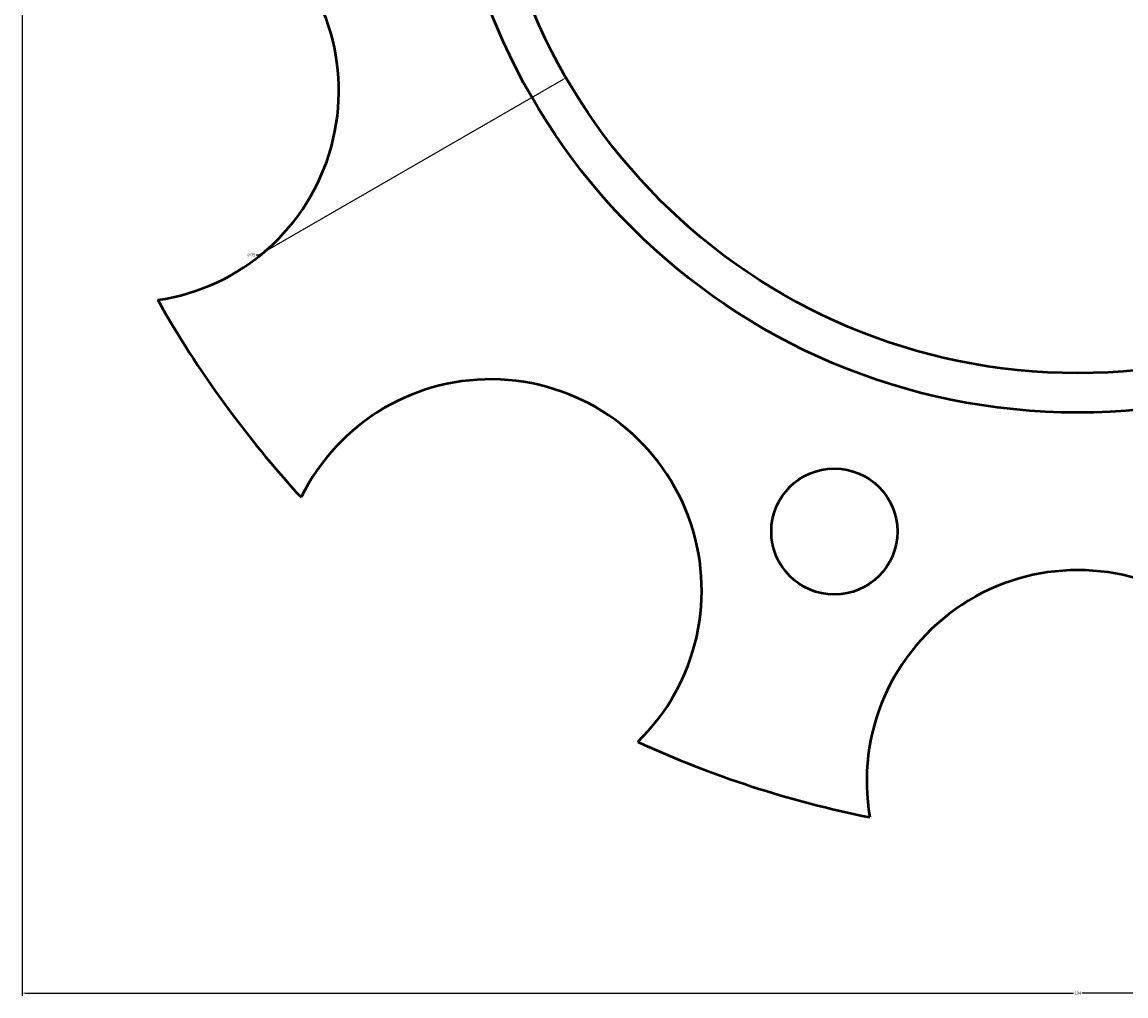
# Model space of a CAD drawing. Units: inches. Extents: x -62 to 104, y -63 to 91.
# Tile 1 of 4: x -42 to 29, y -63 to -1. Entities that reach past the tile are written whole.
import ezdxf

# ---------------------------------------------------------------- set-up
doc = ezdxf.new("R2010")
doc.units = ezdxf.units.IN
doc.header["$MEASUREMENT"] = 0
doc.layers.add('M-DIMS', color=2, linetype='Continuous', lineweight=18)
doc.layers.add('M-OUTL', color=7, linetype='Continuous', lineweight=50)
doc.styles.get("Standard").update_dxf_attribs({"font": 'arial.ttf'})
doc.dimstyles.get("Standard").update_dxf_attribs({"dimtxt": 0.18, "dimasz": 0.18, "dimexe": 0.18, "dimexo": 0.0625, "dimgap": 0.09, "dimtad": 0, "dimtih": 1, "dimtoh": 1, "dimdec": 4, "dimzin": 0, "dimdsep": 46, "dimtxsty": 'Standard', "dimcen": 0.09, "dimadec": 0, "dimazin": 0, "dimtfac": 1, "dimtdec": 4, "dimtofl": 0, "dimtmove": 0, "dimatfit": 3, "dimfxl": 1, "dimtolj": 1, "dimtzin": 0, "dimarcsym": 0})

# ---------------------------------------------------------------- blocks, each defined once
blk = doc.blocks.new('BOLT-HOLE-D8')
blk.add_circle((4, 4), 4)
blk = doc.blocks.new('*D2')
at = {"layer": 'Defpoints', "color": 0, "transparency": 16777216}
for p in [(-41.548, 13.739), (92.452, 13.739), (92.452, -63.102)]:
    blk.add_point(p, dxfattribs=at)
at = {"layer": 'M-DIMS', "color": 0, "lineweight": -2, "transparency": 16777216}
for p, q in [((-41.548, 13.677), (-41.548, -63.282)), ((92.452, 13.677), (92.452, -63.282)), ((-41.368, -63.102), (25.172, -63.102)), ((92.272, -63.102), (25.732, -63.102))]:
    blk.add_line(p, q, dxfattribs=at)
at = {"layer": 'M-DIMS', "color": 0, "transparency": 16777216}
for points in [[(-41.368, -63.072), (-41.368, -63.132), (-41.548, -63.102)], [(92.272, -63.072), (92.272, -63.132), (92.452, -63.102)]]:
    blk.add_solid(points, dxfattribs=at)
at = {"layer": 'M-DIMS', "color": 0, "transparency": 16777216, "insert": (25.452, -63.102), "char_height": 0.18, "attachment_point": 5}
blk.add_mtext('\\A1;134', dxfattribs=at)
blk = doc.blocks.new('*D9')
at = {"layer": 'Defpoints', "color": 0, "transparency": 16777216}
for p in [(57.928, 32.489), (-7.024, -5.011)]:
    blk.add_point(p, dxfattribs=at)
at = {"layer": 'M-DIMS', "color": 0, "lineweight": -2, "transparency": 16777216}
for p, q in [((25.362, 13.739), (25.542, 13.739)), ((25.452, 13.649), (25.452, 13.829)), ((-26.509, -16.261), (-7.18, -5.101)), ((-26.689, -16.261), (-26.509, -16.261))]:
    blk.add_line(p, q, dxfattribs=at)
at = {"layer": 'M-DIMS', "color": 0, "transparency": 16777216}
blk.add_solid([(-7.195, -5.075), (-7.165, -5.127), (-7.024, -5.011)], dxfattribs=at)
at = {"layer": 'M-DIMS', "color": 0, "transparency": 16777216, "insert": (-27.007, -16.261), "char_height": 0.18, "attachment_point": 5}
blk.add_mtext('\\A1;∅75', dxfattribs=at)

msp = doc.modelspace()

# ---------------------------------------------------------------- linework, layer by layer
at = {"layer": 'M-OUTL'}
for radius in [40, 37.5]:
    msp.add_circle((25.452, 13.739), radius, dxfattribs=at)
for centre, radius, start, end in [((-34.845, -5.852), 13.4, 278.17695, 117.82305), ((25.452, 13.739), 67, 209.36555, 222.63445), ((-11.814, -37.552), 13.4, 314.17695, 153.82305), ((25.452, -49.661), 13.4, 350.17695, 189.82305), ((25.452, 13.739), 67, 245.36555, 258.63445)]:
    msp.add_arc(centre, radius, start, end, dxfattribs=at)

# ---------------------------------------------------------------- block references
msp.add_blockref('BOLT-HOLE-D8', (6.001, -37.814), dxfattribs=at)

# ---------------------------------------------------------------- dimensions: what is measured, and where the dimension line sits
at = {"layer": 'M-DIMS'}
dim = msp.add_diameter_dim_2p(p1=(57.928, 32.489), p2=(-7.024, -5.011), dimstyle='Standard', override={"dimdec": 0, "dimlfac": 1, "dimrnd": 0, "dimzin": 0, "dimdsep": 46, "dimlunit": 2}, dxfattribs=at)
dim.commit()
dim.dimension.update_dxf_attribs({"geometry": '*D9', "text_midpoint": (-27.007, -16.261), "dimtype": 163})
dim = msp.add_linear_dim(base=(92.452, -63.102), p1=(-41.548, 13.739), p2=(92.452, 13.739), dimstyle='Standard', override={"dimdec": 0, "dimlfac": 1, "dimrnd": 0, "dimzin": 0, "dimdsep": 46, "dimlunit": 2}, dxfattribs=at)
dim.commit()
dim.dimension.update_dxf_attribs({"geometry": '*D2', "text_midpoint": (25.452, -63.102)})

doc.saveas('drawing.dxf')
